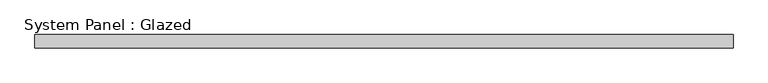
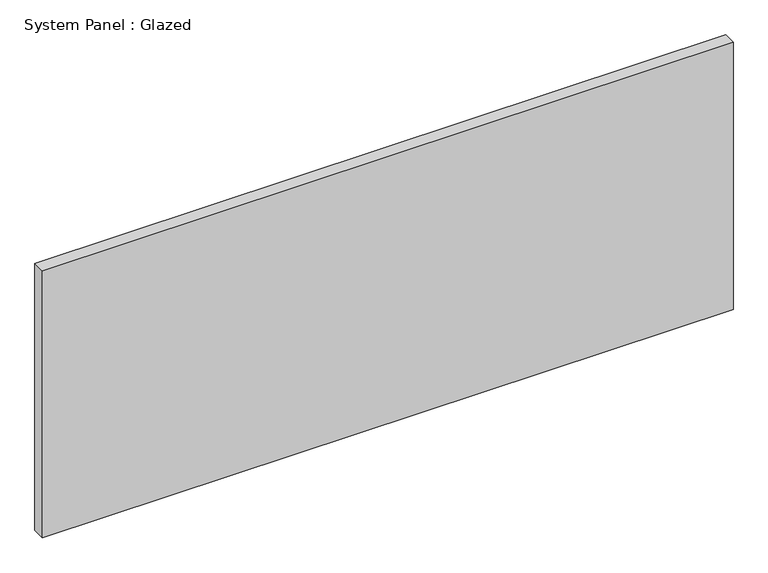
"""IFC4 building model written with IfcOpenShell, lengths in millimetres: plate geometry, System Panel : Glazed."""

from ifc_helpers import new_model, si_unit, origin, origin_with_axes, place, context, project, spatial, polyline, outline, extrude, source, transform, mapped, element, save


def system_panel_glazed_1ceb456a(model_context):
    return source(origin(), model_context, "Body", "SweptSolid", [
        extrude(outline(polyline([(667.2791666, 19.05), (-667.2791666, 19.05), (-667.2791666, 44.45), (667.2791666, 44.45), (667.2791666, 19.05)])), origin_with_axes(), (0.0, 0.0, 1.0), 546.1),
    ])


if __name__ == "__main__":
    model = new_model("IFC4")
    model_context = context("Model", 3, world=origin())
    ifc_project = project(units=[si_unit("LENGTHUNIT", "METRE", prefix="MILLI")], contexts=[model_context])
    site = spatial("IfcSite", under=ifc_project)
    building = spatial("IfcBuilding", under=site)
    placement = place(None, origin())
    system_panel_glazed_shape = system_panel_glazed_1ceb456a(model_context)
    element("IfcPlate", 1, ObjectType="System Panel : Glazed", at=placement, inside=building, context=model_context, shape_type="MappedRepresentation", body=[
        mapped(system_panel_glazed_shape, transform((0.0, 0.0, 0.0), x_axis=(1.0, 0.0, 0.0), y_axis=(0.0, 1.0, 0.0), z_axis=(0.0, 0.0, 1.0))),
    ])
    save(model, "model.ifc")

# Revit data of these elements
# Type "System Panel : Glazed"
#   Construction Type Id = "GSP4R"
#   Analytic Construction = "1/8 in Pilkington single glazing"
#   Visual Light Transmittance = 0.9
#   Solar Heat Gain Coefficient = 0.86
#   Heat Transfer Coefficient (U) = 1.18115 BTU/(h·ft²·°F)
#   Define Thermal Properties by = 1
# Element 1 (IfcPlate, "System Panel : Glazed")
#   Materials on its faces: "Glass"
# Materials
#   "Glass": class "Glass", colour RGB 0 128 192, transparency 0.75, Description = "Soda Lime Glass", Cost = 0
